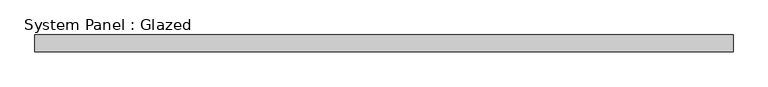
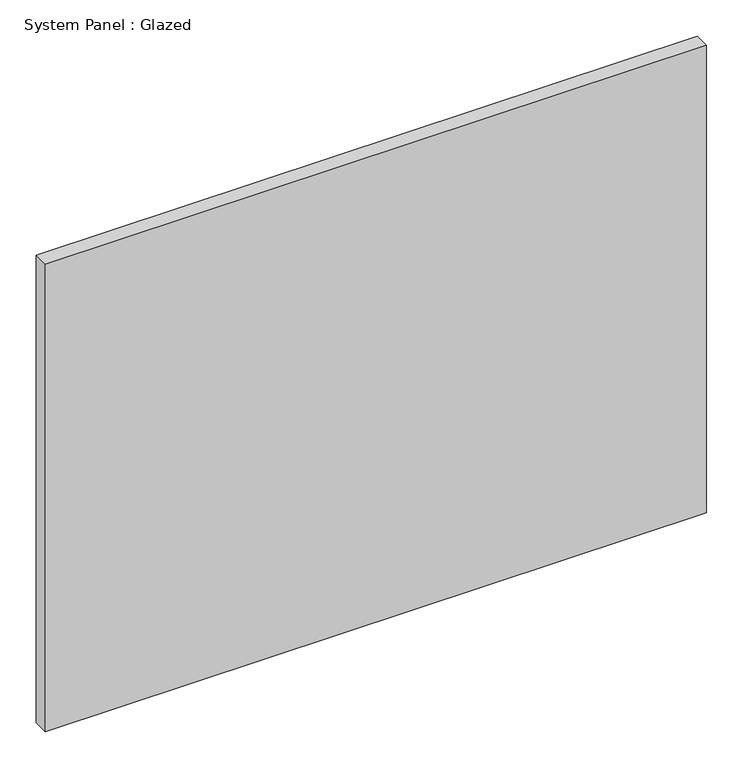
"""IFC4 building model written with IfcOpenShell, lengths in millimetres: plate geometry, System Panel : Glazed."""

from ifc_helpers import new_model, si_unit, origin, origin_with_axes, place, context, project, spatial, polyline, outline, extrude, source, transform, mapped, element, save


def system_panel_glazed_cfce8111(model_context):
    return source(origin(), model_context, "Body", "SweptSolid", [
        extrude(outline(polyline([(527.05, 19.05), (-527.05, 19.05), (-527.05, 44.45), (527.05, 44.45), (527.05, 19.05)])), origin_with_axes(), (0.0, 0.0, 1.0), 787.4),
    ])


if __name__ == "__main__":
    model = new_model("IFC4")
    model_context = context("Model", 3, world=origin())
    ifc_project = project(units=[si_unit("LENGTHUNIT", "METRE", prefix="MILLI")], contexts=[model_context])
    site = spatial("IfcSite", under=ifc_project)
    building = spatial("IfcBuilding", under=site)
    placement = place(None, origin())
    system_panel_glazed_shape = system_panel_glazed_cfce8111(model_context)
    element("IfcPlate", 1, ObjectType="System Panel : Glazed", at=placement, inside=building, context=model_context, shape_type="MappedRepresentation", body=[
        mapped(system_panel_glazed_shape, transform((0.0, 0.0, 0.0), x_axis=(1.0, 0.0, 0.0), y_axis=(0.0, 1.0, 0.0), z_axis=(0.0, 0.0, 1.0))),
    ])
    save(model, "model.ifc")

# Revit data of these elements
# Type "System Panel : Glazed"
#   Construction Type Id = "GSP4R"
#   Analytic Construction = "1/8 in Pilkington single glazing"
#   Visual Light Transmittance = 0.9
#   Solar Heat Gain Coefficient = 0.86
#   Heat Transfer Coefficient (U) = 1.18115 BTU/(h·ft²·°F)
# Element 1 (IfcPlate, "System Panel : Glazed")
#   Materials on its faces: "Glass"
# Materials
#   "Glass": class "Glass", colour RGB 0 128 192, transparency 0.75, Description = "Soda Lime Glass", Cost = 0
